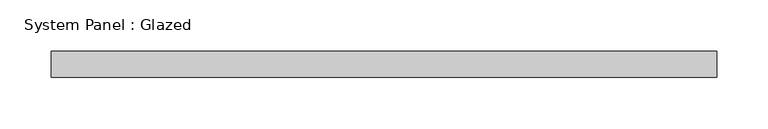
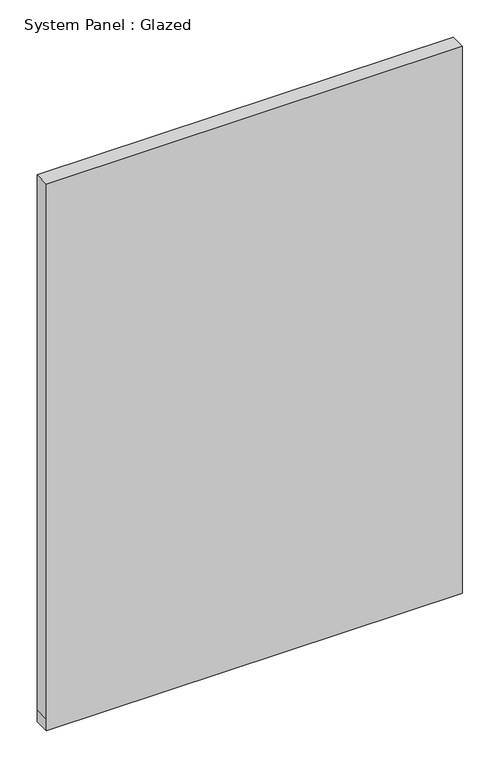
"""IFC4 building model written with IfcOpenShell, lengths in millimetres: plate geometry, System Panel : Glazed."""

from ifc_helpers import new_model, si_unit, frame, origin, place, context, project, spatial, polyline, outline, extrude, source, transform, mapped, element, save


def system_panel_glazed_c0474106(model_context):
    return source(origin(), model_context, "Body", "SweptSolid", [
        extrude(outline(polyline([(0.0, -323.85), (0.0, 323.85), (19.05, 323.85), (900.0180153, 323.85), (900.0180153, -323.85), (19.05, -323.85), (0.0, -323.85)])), frame((0.0, 19.05, 0.0), z_axis=(0.0, 1.0, 0.0), x_axis=(0.0, 0.0, 1.0)), (0.0, 0.0, 1.0), 25.4),
    ])


if __name__ == "__main__":
    model = new_model("IFC4")
    model_context = context("Model", 3, world=origin())
    ifc_project = project(units=[si_unit("LENGTHUNIT", "METRE", prefix="MILLI")], contexts=[model_context])
    site = spatial("IfcSite", under=ifc_project)
    building = spatial("IfcBuilding", under=site)
    placement = place(None, origin())
    system_panel_glazed_shape = system_panel_glazed_c0474106(model_context)
    element("IfcPlate", 1, ObjectType="System Panel : Glazed", at=placement, inside=building, context=model_context, shape_type="MappedRepresentation", body=[
        mapped(system_panel_glazed_shape, transform((0.0, 0.0, 0.0), x_axis=(1.0, 0.0, 0.0), y_axis=(0.0, 1.0, 0.0), z_axis=(0.0, 0.0, 1.0))),
    ])
    save(model, "model.ifc")

# Revit data of these elements
# Type "System Panel : Glazed"
#   Construction Type Id = "GSP4R"
#   Analytic Construction = "1/8 in Pilkington single glazing"
#   Visual Light Transmittance = 0.9
#   Solar Heat Gain Coefficient = 0.86
#   Heat Transfer Coefficient (U) = 1.18115 BTU/(h·ft²·°F)
#   Define Thermal Properties by = 1
# Element 1 (IfcPlate, "System Panel : Glazed")
#   Materials on its faces: "Glass"
# Materials
#   "Glass": class "Glass", colour RGB 0 128 192, transparency 0.75, Description = "Soda Lime Glass", Cost = 0
